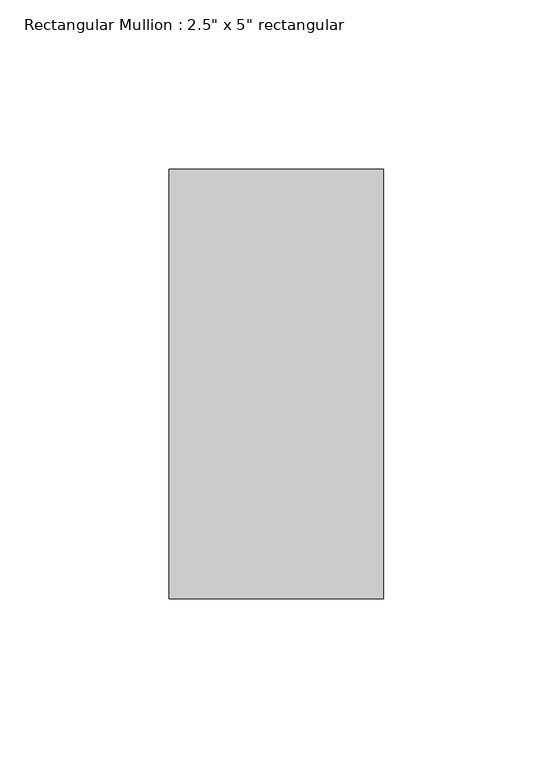
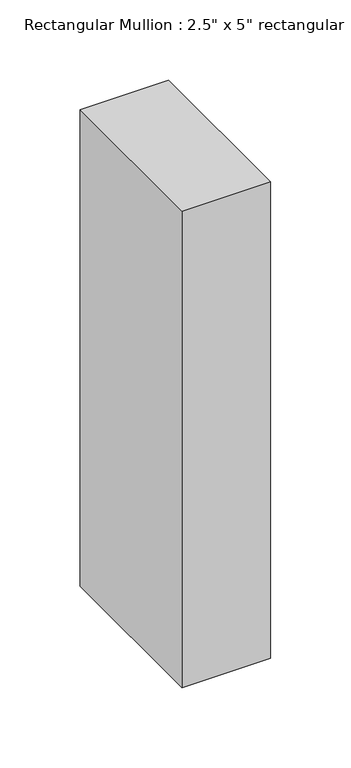
"""IFC4 building model written with IfcOpenShell, lengths in millimetres: member geometry."""

from ifc_helpers import new_model, si_unit, frame, origin, place, context, project, spatial, polyline, outline, extrude, source, transform, mapped, element, save


def member_843225dc(model_context):
    return source(origin(), model_context, "Body", "SweptSolid", [
        extrude(outline(polyline([(0.0, 63.5), (0.0, -63.5), (-63.5, -63.5), (-63.5, 63.5), (0.0, 63.5)])), frame((0.0, 0.0, -361.95), z_axis=(0.0, 0.0, 1.0), x_axis=(1.0, 0.0, 0.0)), (0.0, 0.0, 1.0), 361.95),
    ])


if __name__ == "__main__":
    model = new_model("IFC4")
    model_context = context("Model", 3, world=origin())
    ifc_project = project(units=[si_unit("LENGTHUNIT", "METRE", prefix="MILLI")], contexts=[model_context])
    site = spatial("IfcSite", under=ifc_project)
    building = spatial("IfcBuilding", under=site)
    placement = place(None, origin())
    member_shape = member_843225dc(model_context)
    element("IfcMember", 1, ObjectType="Rectangular Mullion : 2.5\" x 5\" rectangular", at=placement, inside=building, context=model_context, shape_type="MappedRepresentation", body=[
        mapped(member_shape, transform((0.0, 0.0, 0.0), x_axis=(1.0, 0.0, 0.0), y_axis=(0.0, 1.0, 0.0), z_axis=(0.0, 0.0, 1.0))),
    ])
    save(model, "model.ifc")

# Revit data of these elements
# Type "Rectangular Mullion : 2.5\" x 5\" rectangular"
#   built-in parameter 1007304 = 0.416667 (stored number, unit not read)
#   built-in parameter 1007301 = 0.104167 (stored number, unit not read)
#   built-in parameter 1007300 = 0.104167 (stored number, unit not read)
# Element 1 (IfcMember, "Rectangular Mullion : 2.5\" x 5\" rectangular")
#   Materials on its faces: "Aluminum"
# Materials
#   "Aluminum": class "Metal", colour RGB 247 247 247, transparency 0, Description = "Aluminum 6061", Cost = 0
